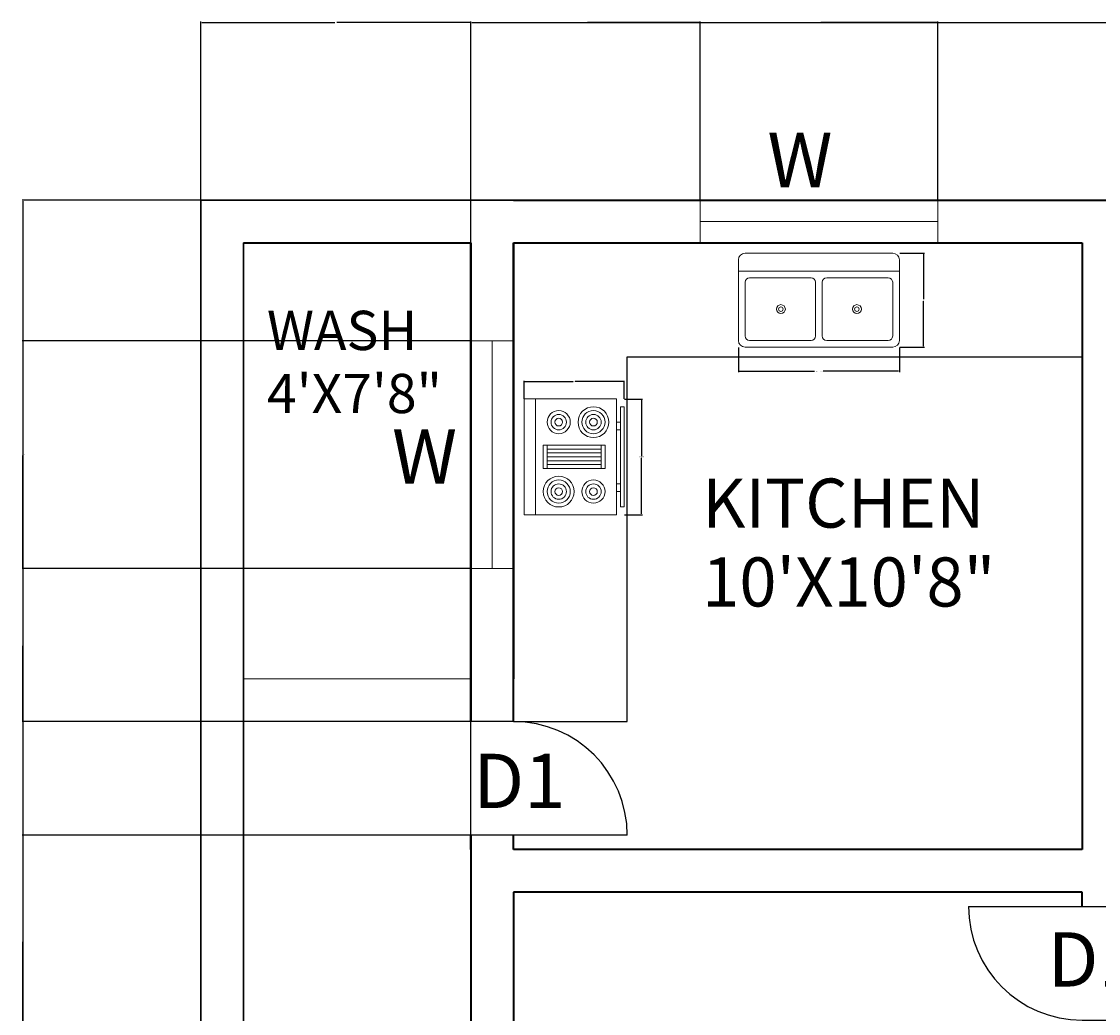
# Model space of a CAD drawing. Units: feet. Extents: x 1889 to 2708, y 1752 to 2375.
# Tile 3 of 5: x 1889 to 2116, y 2166 to 2375. Entities that reach past the tile are written whole.
import ezdxf

# ---------------------------------------------------------------- set-up
doc = ezdxf.new("R2010")
doc.units = ezdxf.units.FT
for name, color, linetype, lineweight in [('A-ANNO-DIMS', 2, 'Continuous', 18), ('A-ANNO-TEXT', 7, 'Continuous', 18), ('A-AREA-IDEN', 7, 'Continuous', 18), ('A-DOOR', 3, 'Continuous', 25), ('A-EQPM', 9, 'Continuous', 18), ('A-FLOR-CASE', 9, 'Continuous', 25), ('A-FLOR-FIXT', 8, 'Continuous', 18), ('A-GLAZ', 4, 'Continuous', 18), ('A-WALL', 7, 'Continuous', 35), ('C-PROP', 7, 'Continuous', 30), ('C-SITE', 94, 'Continuous', 18)]:
    doc.layers.add(name, color=color, linetype=linetype, lineweight=lineweight)
doc.styles.get("Standard").update_dxf_attribs({"font": 'arial.ttf'})
doc.dimstyles.get("Standard").update_dxf_attribs({"dimtxt": 0.18, "dimasz": 0.18, "dimexe": 0.18, "dimexo": 0.0625, "dimgap": 0.09, "dimtad": 0, "dimtih": 1, "dimtoh": 1, "dimdec": 4, "dimzin": 0, "dimdsep": 46, "dimtxsty": 'Standard', "dimcen": 0.09, "dimadec": 0, "dimazin": 0, "dimtfac": 1, "dimtdec": 4, "dimtofl": 0, "dimtmove": 0, "dimatfit": 3, "dimfxl": 1, "dimtolj": 1, "dimtzin": 0, "dimarcsym": 0})

# ---------------------------------------------------------------- blocks, each defined once
blk = doc.blocks.new('Range-Oven - 30 in top')
for p, q in [((0, -3), (30, -3)), ((12, -6), (18, -6)), ((13, -20), (13, -6)), ((14, -6), (14, -20)), ((15, -20), (15, -6)), ((16, -6), (16, -20)), ((17, -20), (17, -6)), ((18, -20), (12, -20)), ((6, -24), (6, -25)), ((8, -25), (8, -24)), ((22, -25), (22, -24)), ((24, -24), (24, -25))]:
    blk.add_line(p, q)
for points in [[(0, -24), (0, 0), (30, 0), (30, -24)], [(12, -21), (12, -5), (18, -5), (18, -21)], [(2, -26), (2, -25), (28, -25), (28, -26)]]:
    blk.add_lwpolyline(points, close=True)
for centre, radius in [((6, -9), 4), ((6, -9), 3), ((6, -9), 2), ((6, -9), 1), ((24, -9), 3), ((24, -9), 2), ((24, -9), 1), ((6, -18), 3), ((6, -18), 2), ((24, -18), 4), ((24, -18), 3), ((24, -18), 2), ((6, -18), 1), ((24, -18), 1)]:
    blk.add_circle(centre, radius)
blk = doc.blocks.new('Sink-double - 36 in top')
for p, q in [((-18, -4), (18, -4)), ((-0.75, -18.5), (-0.75, -6.5)), ((0.75, -6.5), (0.75, -18.5))]:
    blk.add_line(p, q)
for points in [[(-16.5, 0), (16.5, 0)], [(-18, -19.5), (-18, -1.5)], [(18, -1.5), (18, -19.5)], [(-16.5, -18.5), (-16.5, -6.5)], [(-15.5, -5.5), (-1.75, -5.5)], [(1.75, -5.5), (15.5, -5.5)], [(16.5, -6.5), (16.5, -18.5)], [(16.5, -21), (-16.5, -21)], [(-1.75, -19.5), (-15.5, -19.5)], [(15.5, -19.5), (1.75, -19.5)]]:
    blk.add_lwpolyline(points)
for centre, radius in [((-8.5, -12.5), 1), ((-8.5, -12.5), 0.5), ((8.5, -12.5), 1), ((8.5, -12.5), 0.5)]:
    blk.add_circle(centre, radius)
for centre, radius, start, end in [((-16.5, -1.5), 1.5, 90, 180), ((16.5, -1.5), 1.5, 0, 90), ((-15.5, -6.5), 1, 90, 180), ((-1.75, -6.5), 1, 0, 90), ((1.75, -6.5), 1, 90, 180), ((15.5, -6.5), 1, 0, 90), ((-15.5, -18.5), 1, 180, 270), ((-1.75, -18.5), 1, 270, 0), ((1.75, -18.5), 1, 180, 270), ((15.5, -18.5), 1, 270, 0), ((-16.5, -19.5), 1.5, 180, 270), ((16.5, -19.5), 1.5, 270, 0)]:
    blk.add_arc(centre, radius, start, end)
blk = doc.blocks.new('DOOR-SWING-24')
for p, q in [((9, 24), (0, 24)), ((33, 0), (0, 0))]:
    blk.add_line(p, q)
blk.add_arc((9, 0), 24, 0, 90)
blk = doc.blocks.new('*D27')
at = {"layer": 'A-ANNO-DIMS', "color": 0, "lineweight": -2, "transparency": 16777216}
for p, q in [((2016.29, 2295.67), (2020.07, 2295.67)), ((2019.89, 2295.49), (2019.89, 2283.65)), ((2019.89, 2271.43), (2019.89, 2283.28)), ((2016.29, 2271.25), (2020.07, 2271.25))]:
    blk.add_line(p, q, dxfattribs=at)
at = {"layer": 'A-ANNO-DIMS', "color": 0, "transparency": 16777216}
for points in [[(2019.86, 2295.49), (2019.92, 2295.49), (2019.89, 2295.67)], [(2019.86, 2271.43), (2019.92, 2271.43), (2019.89, 2271.25)]]:
    blk.add_solid(points, dxfattribs=at)
at = {"layer": 'Defpoints', "color": 0, "transparency": 16777216}
for p in [(2016.23, 2295.67), (2019.89, 2295.67), (2016.23, 2271.25)]:
    blk.add_point(p, dxfattribs=at)
at = {"layer": 'A-ANNO-DIMS', "color": 0, "transparency": 16777216, "insert": (2019.89, 2283.46), "char_height": 0.18, "attachment_point": 5}
blk.add_mtext('\\A1;HOB 24', dxfattribs=at)
blk = doc.blocks.new('*D28')
at = {"layer": 'A-ANNO-DIMS', "color": 0, "lineweight": -2, "transparency": 16777216}
for p, q in [((1995.07, 2295.73), (1995.07, 2299.51)), ((1995.25, 2299.33), (2005.44, 2299.33)), ((2016.05, 2299.33), (2005.85, 2299.33)), ((2016.23, 2295.73), (2016.23, 2299.51))]:
    blk.add_line(p, q, dxfattribs=at)
at = {"layer": 'A-ANNO-DIMS', "color": 0, "transparency": 16777216}
for points in [[(1995.25, 2299.36), (1995.25, 2299.3), (1995.07, 2299.33)], [(2016.05, 2299.36), (2016.05, 2299.3), (2016.23, 2299.33)]]:
    blk.add_solid(points, dxfattribs=at)
at = {"layer": 'Defpoints', "color": 0, "transparency": 16777216}
for p in [(1995.07, 2299.33), (1995.07, 2295.67), (2016.23, 2295.67)]:
    blk.add_point(p, dxfattribs=at)
at = {"layer": 'A-ANNO-DIMS', "color": 0, "transparency": 16777216, "insert": (2005.65, 2299.33), "char_height": 0.18, "attachment_point": 5}
blk.add_mtext('\\A1;21', dxfattribs=at)
blk = doc.blocks.new('*D33')
at = {"layer": 'A-ANNO-DIMS', "color": 0, "lineweight": -2, "transparency": 16777216}
for p, q in [((2040.31, 2306.55), (2040.31, 2301.34)), ((2074.29, 2306.55), (2074.29, 2301.34)), ((2040.49, 2301.52), (2056.4, 2301.52)), ((2074.11, 2301.52), (2058.21, 2301.52))]:
    blk.add_line(p, q, dxfattribs=at)
at = {"layer": 'A-ANNO-DIMS', "color": 0, "transparency": 16777216}
for points in [[(2040.49, 2301.55), (2040.49, 2301.49), (2040.31, 2301.52)], [(2074.11, 2301.55), (2074.11, 2301.49), (2074.29, 2301.52)]]:
    blk.add_solid(points, dxfattribs=at)
at = {"layer": 'Defpoints', "color": 0, "transparency": 16777216}
for p in [(2040.31, 2306.61), (2074.29, 2306.61), (2074.29, 2301.52)]:
    blk.add_point(p, dxfattribs=at)
at = {"layer": 'A-ANNO-DIMS', "color": 0, "transparency": 16777216, "insert": (2057.3, 2301.52), "char_height": 0.18, "attachment_point": 5}
blk.add_mtext('\\A1;TWIN SINK 34', dxfattribs=at)
blk = doc.blocks.new('*D34')
at = {"layer": 'A-ANNO-DIMS', "color": 0, "lineweight": -2, "transparency": 16777216}
for p, q in [((2074.35, 2326.44), (2079.57, 2326.44)), ((2079.39, 2326.26), (2079.39, 2316.71)), ((2079.39, 2306.79), (2079.39, 2316.34)), ((2074.35, 2306.61), (2079.57, 2306.61))]:
    blk.add_line(p, q, dxfattribs=at)
at = {"layer": 'A-ANNO-DIMS', "color": 0, "transparency": 16777216}
for points in [[(2079.36, 2326.26), (2079.42, 2326.26), (2079.39, 2326.44)], [(2079.36, 2306.79), (2079.42, 2306.79), (2079.39, 2306.61)]]:
    blk.add_solid(points, dxfattribs=at)
at = {"layer": 'Defpoints', "color": 0, "transparency": 16777216}
for p in [(2074.29, 2326.44), (2079.39, 2326.44), (2074.29, 2306.61)]:
    blk.add_point(p, dxfattribs=at)
at = {"layer": 'A-ANNO-DIMS', "color": 0, "transparency": 16777216, "insert": (2079.39, 2316.53), "char_height": 0.18, "attachment_point": 5}
blk.add_mtext('\\A1;20', dxfattribs=at)
blk = doc.blocks.new('*D35')
at = {"layer": 'A-ANNO-DIMS', "color": 0, "lineweight": -2, "transparency": 16777216}
for p, q in [((1926.86, 2337.66), (1926.86, 2375.33)), ((1983.86, 2328.66), (1983.86, 2375.33)), ((1927.04, 2375.15), (1955.15, 2375.15)), ((1983.68, 2375.15), (1955.58, 2375.15))]:
    blk.add_line(p, q, dxfattribs=at)
at = {"layer": 'A-ANNO-DIMS', "color": 0, "transparency": 16777216}
for points in [[(1927.04, 2375.18), (1927.04, 2375.12), (1926.86, 2375.15)], [(1983.68, 2375.18), (1983.68, 2375.12), (1983.86, 2375.15)]]:
    blk.add_solid(points, dxfattribs=at)
at = {"layer": 'Defpoints', "color": 0, "transparency": 16777216}
for p in [(1983.86, 2375.15), (1926.86, 2337.6), (1983.86, 2328.6)]:
    blk.add_point(p, dxfattribs=at)
at = {"layer": 'A-ANNO-DIMS', "color": 0, "transparency": 16777216, "insert": (1955.36, 2375.15), "char_height": 0.18, "attachment_point": 5}
blk.add_mtext('\\A1;57', dxfattribs=at)
blk = doc.blocks.new('*D36')
at = {"layer": 'A-ANNO-DIMS', "color": 0, "lineweight": -2, "transparency": 16777216}
for p, q in [((1983.86, 2328.66), (1983.86, 2375.33)), ((2032.22, 2337.66), (2032.22, 2375.33)), ((1984.04, 2375.15), (2007.64, 2375.15)), ((2032.04, 2375.15), (2008.44, 2375.15))]:
    blk.add_line(p, q, dxfattribs=at)
at = {"layer": 'A-ANNO-DIMS', "color": 0, "transparency": 16777216}
for points in [[(1984.04, 2375.18), (1984.04, 2375.12), (1983.86, 2375.15)], [(2032.04, 2375.18), (2032.04, 2375.12), (2032.22, 2375.15)]]:
    blk.add_solid(points, dxfattribs=at)
at = {"layer": 'Defpoints', "color": 0, "transparency": 16777216}
for p in [(2032.22, 2375.15), (2032.22, 2337.6), (1983.86, 2328.6)]:
    blk.add_point(p, dxfattribs=at)
at = {"layer": 'A-ANNO-DIMS', "color": 0, "transparency": 16777216, "insert": (2008.04, 2375.15), "char_height": 0.18, "attachment_point": 5}
blk.add_mtext('\\A1;48.35', dxfattribs=at)
blk = doc.blocks.new('*D37')
at = {"layer": 'A-ANNO-DIMS', "color": 0, "lineweight": -2, "transparency": 16777216}
for p, q in [((2032.22, 2337.66), (2032.22, 2375.33)), ((2082.41, 2337.66), (2082.41, 2375.33)), ((2032.4, 2375.15), (2056.92, 2375.15)), ((2082.23, 2375.15), (2057.71, 2375.15))]:
    blk.add_line(p, q, dxfattribs=at)
at = {"layer": 'A-ANNO-DIMS', "color": 0, "transparency": 16777216}
for points in [[(2032.4, 2375.18), (2032.4, 2375.12), (2032.22, 2375.15)], [(2082.23, 2375.18), (2082.23, 2375.12), (2082.41, 2375.15)]]:
    blk.add_solid(points, dxfattribs=at)
at = {"layer": 'Defpoints', "color": 0, "transparency": 16777216}
for p in [(2082.41, 2375.15), (2032.22, 2337.6), (2082.41, 2337.6)]:
    blk.add_point(p, dxfattribs=at)
at = {"layer": 'A-ANNO-DIMS', "color": 0, "transparency": 16777216, "insert": (2057.31, 2375.15), "char_height": 0.18, "attachment_point": 5}
blk.add_mtext('\\A1;50.19', dxfattribs=at)
blk = doc.blocks.new('*D38')
at = {"layer": 'A-ANNO-DIMS', "color": 0, "lineweight": -2, "transparency": 16777216}
for p, q in [((2082.41, 2337.66), (2082.41, 2375.33)), ((2344.63, 2337.66), (2344.63, 2375.33)), ((2082.59, 2375.15), (2213.05, 2375.15)), ((2344.45, 2375.15), (2213.98, 2375.15))]:
    blk.add_line(p, q, dxfattribs=at)
at = {"layer": 'A-ANNO-DIMS', "color": 0, "transparency": 16777216}
for points in [[(2082.59, 2375.18), (2082.59, 2375.12), (2082.41, 2375.15)], [(2344.45, 2375.18), (2344.45, 2375.12), (2344.63, 2375.15)]]:
    blk.add_solid(points, dxfattribs=at)
at = {"layer": 'Defpoints', "color": 0, "transparency": 16777216}
for p in [(2344.63, 2375.15), (2082.41, 2337.6), (2344.63, 2337.6)]:
    blk.add_point(p, dxfattribs=at)
at = {"layer": 'A-ANNO-DIMS', "color": 0, "transparency": 16777216, "insert": (2213.52, 2375.15), "char_height": 0.18, "attachment_point": 5}
blk.add_mtext('\\A1;262.23', dxfattribs=at)
blk = doc.blocks.new('*D46')
at = {"layer": 'A-ANNO-DIMS', "color": 0, "lineweight": -2, "transparency": 16777216}
for p, q in [((1926.8, 2337.6), (1889.13, 2337.6)), ((1889.31, 2337.42), (1889.31, 2121.28)), ((1889.31, 1904.78), (1889.31, 2120.92)), ((1983.8, 1904.6), (1889.13, 1904.6))]:
    blk.add_line(p, q, dxfattribs=at)
at = {"layer": 'A-ANNO-DIMS', "color": 0, "transparency": 16777216}
for points in [[(1889.28, 2337.42), (1889.34, 2337.42), (1889.31, 2337.6)], [(1889.28, 1904.78), (1889.34, 1904.78), (1889.31, 1904.6)]]:
    blk.add_solid(points, dxfattribs=at)
at = {"layer": 'Defpoints', "color": 0, "transparency": 16777216}
for p in [(1889.31, 2337.6), (1926.86, 2337.6), (1983.86, 1904.6)]:
    blk.add_point(p, dxfattribs=at)
at = {"layer": 'A-ANNO-DIMS', "color": 0, "transparency": 16777216, "insert": (1889.31, 2121.1), "char_height": 0.18, "attachment_point": 5}
blk.add_mtext('\\A1;433', dxfattribs=at)
blk = doc.blocks.new('*D48')
at = {"layer": 'A-ANNO-DIMS', "color": 0, "lineweight": -2, "transparency": 16777216}
for p, q in [((1983.86, 1820.66), (1983.86, 2375.33)), ((2432.86, 1820.66), (2432.86, 2375.33)), ((1984.04, 2375.15), (2208.07, 2375.15)), ((2432.68, 2375.15), (2208.66, 2375.15))]:
    blk.add_line(p, q, dxfattribs=at)
at = {"layer": 'A-ANNO-DIMS', "color": 0, "transparency": 16777216}
for points in [[(1984.04, 2375.18), (1984.04, 2375.12), (1983.86, 2375.15)], [(2432.68, 2375.18), (2432.68, 2375.12), (2432.86, 2375.15)]]:
    blk.add_solid(points, dxfattribs=at)
at = {"layer": 'Defpoints', "color": 0, "transparency": 16777216}
for p in [(2432.86, 2375.15), (1983.86, 1820.6), (2432.86, 1820.6)]:
    blk.add_point(p, dxfattribs=at)
at = {"layer": 'A-ANNO-DIMS', "color": 0, "transparency": 16777216, "insert": (2208.36, 2375.15), "char_height": 0.18, "attachment_point": 5}
blk.add_mtext('\\A1;449', dxfattribs=at)
blk = doc.blocks.new('*D55')
at = {"layer": 'A-ANNO-DIMS', "color": 0, "lineweight": -2, "transparency": 16777216}
for p, q in [((1983.8, 2203.6), (1889.13, 2203.6)), ((1889.31, 2203.42), (1889.31, 2181.48)), ((1889.31, 2159.18), (1889.31, 2181.12)), ((1983.8, 2159), (1889.13, 2159))]:
    blk.add_line(p, q, dxfattribs=at)
at = {"layer": 'A-ANNO-DIMS', "color": 0, "transparency": 16777216}
for points in [[(1889.28, 2203.42), (1889.34, 2203.42), (1889.31, 2203.6)], [(1889.28, 2159.18), (1889.34, 2159.18), (1889.31, 2159)]]:
    blk.add_solid(points, dxfattribs=at)
at = {"layer": 'Defpoints', "color": 0, "transparency": 16777216}
for p in [(1889.31, 2203.6), (1983.86, 2203.6), (1983.86, 2159)]:
    blk.add_point(p, dxfattribs=at)
at = {"layer": 'A-ANNO-DIMS', "color": 0, "transparency": 16777216, "insert": (1889.31, 2181.3), "char_height": 0.18, "attachment_point": 5}
blk.add_mtext('\\A1;44.6', dxfattribs=at)
blk = doc.blocks.new('*D56')
at = {"layer": 'A-ANNO-DIMS', "color": 0, "lineweight": -2, "transparency": 16777216}
for p, q in [((1983.8, 2259.92), (1889.13, 2259.92)), ((1889.31, 2259.74), (1889.31, 2243.94)), ((1889.31, 2227.78), (1889.31, 2243.58)), ((1983.8, 2227.6), (1889.13, 2227.6))]:
    blk.add_line(p, q, dxfattribs=at)
at = {"layer": 'A-ANNO-DIMS', "color": 0, "transparency": 16777216}
for points in [[(1889.28, 2259.74), (1889.34, 2259.74), (1889.31, 2259.92)], [(1889.28, 2227.78), (1889.34, 2227.78), (1889.31, 2227.6)]]:
    blk.add_solid(points, dxfattribs=at)
at = {"layer": 'Defpoints', "color": 0, "transparency": 16777216}
for p in [(1889.31, 2259.92), (1983.86, 2259.92), (1983.86, 2227.6)]:
    blk.add_point(p, dxfattribs=at)
at = {"layer": 'A-ANNO-DIMS', "color": 0, "transparency": 16777216, "insert": (1889.31, 2243.76), "char_height": 0.18, "attachment_point": 5}
blk.add_mtext('\\A1;32.32', dxfattribs=at)
blk = doc.blocks.new('*D57')
at = {"layer": 'A-ANNO-DIMS', "color": 0, "lineweight": -2, "transparency": 16777216}
for p, q in [((1983.8, 2307.98), (1889.13, 2307.98)), ((1889.31, 2307.8), (1889.31, 2284.13)), ((1889.31, 2260.1), (1889.31, 2283.77)), ((1983.8, 2259.92), (1889.13, 2259.92))]:
    blk.add_line(p, q, dxfattribs=at)
at = {"layer": 'A-ANNO-DIMS', "color": 0, "transparency": 16777216}
for points in [[(1889.28, 2307.8), (1889.34, 2307.8), (1889.31, 2307.98)], [(1889.28, 2260.1), (1889.34, 2260.1), (1889.31, 2259.92)]]:
    blk.add_solid(points, dxfattribs=at)
at = {"layer": 'Defpoints', "color": 0, "transparency": 16777216}
for p in [(1889.31, 2307.98), (1983.86, 2307.98), (1983.86, 2259.92)]:
    blk.add_point(p, dxfattribs=at)
at = {"layer": 'A-ANNO-DIMS', "color": 0, "transparency": 16777216, "insert": (1889.31, 2283.95), "char_height": 0.18, "attachment_point": 5}
blk.add_mtext('\\A1;48.06', dxfattribs=at)

msp = doc.modelspace()

# ---------------------------------------------------------------- linework, layer by layer
at = {"layer": 'A-FLOR-CASE'}
for p, q in [((2016.8644, 2304.5988), (2112.8644, 2304.5988)), ((2016.8644, 2227.5988), (2016.8644, 2304.5988)), ((1992.8644, 2227.5988), (2016.8644, 2227.5988))]:
    msp.add_line(p, q, dxfattribs=at)
at = {"layer": 'A-GLAZ'}
for p, q in [((2032.217, 2337.5988), (2032.217, 2328.5988)), ((2082.4064, 2337.5988), (2082.4064, 2328.5988)), ((2032.217, 2333.0988), (2082.4064, 2333.0988)), ((1983.8644, 2307.9791), (1992.8644, 2307.9791)), ((1988.3644, 2307.9791), (1988.3644, 2259.9212)), ((1983.8644, 2259.9212), (1992.8644, 2259.9212))]:
    msp.add_line(p, q, dxfattribs=at)
at = {"layer": 'A-WALL'}
for p, q in [((1992.8644, 2337.5988), (2669.8644, 2337.5988)), ((1935.8644, 2328.5988), (1983.8644, 2328.5988)), ((1983.8644, 2328.5988), (1983.8644, 2236.5988)), ((1983.8644, 2227.5988), (1983.8644, 2328.5988)), ((1992.8644, 2328.5988), (1992.8644, 2236.5988)), ((1992.8644, 2328.5988), (2112.8644, 2328.5988)), ((1992.8644, 2227.5988), (1992.8644, 2328.5988)), ((2112.8644, 2328.5988), (2112.8644, 2200.5988)), ((1983.8644, 2236.5988), (1983.8644, 2227.5988)), ((1983.8644, 2236.5988), (1983.8644, 2227.5988)), ((1983.8644, 2236.5988), (1983.8644, 2227.5988)), ((1983.8644, 2200.5988), (1983.8644, 2203.5988)), ((1983.8644, 2203.5988), (1983.8644, 1904.5988)), ((1983.8644, 2203.5988), (1983.8644, 1974.5988)), ((1983.8644, 2203.5988), (1983.8644, 2039.5988)), ((1992.8644, 2200.5988), (1992.8644, 2203.5988)), ((2112.8644, 2200.5988), (1992.8644, 2200.5988)), ((2112.8644, 2191.5988), (1992.8644, 2191.5988)), ((1992.8644, 2191.5988), (1992.8644, 2039.5988)), ((2112.8644, 2188.5988), (2112.8644, 2191.5988))]:
    msp.add_line(p, q, dxfattribs=at)
at = {"layer": 'C-PROP'}
for p, q in [((1926.8644, 2337.5988), (2669.8644, 2337.5988)), ((1926.8644, 2236.5988), (1926.8644, 2337.5988)), ((1935.8644, 1811.5988), (1935.8644, 2328.5988)), ((1926.8644, 2236.5988), (1926.8644, 1811.5988))]:
    msp.add_line(p, q, dxfattribs=at)
at = {"layer": 'C-SITE'}
msp.add_line((1983.8644, 2236.5988), (1935.8644, 2236.5988), dxfattribs=at)

# ---------------------------------------------------------------- block references
at = {"layer": 'A-DOOR'}
msp.add_blockref('DOOR-SWING-24', (1983.864, 2203.599), dxfattribs=at)
at = {"layer": 'A-DOOR', "rotation": 180}
msp.add_blockref('DOOR-SWING-24', (2121.8649, 2188.5986), dxfattribs=at)
at = {"layer": 'A-EQPM', "xscale": 0.8139749521299275, "yscale": 0.8139749521299275, "zscale": 0.8139749521299275, "rotation": 90}
msp.add_blockref('Range-Oven - 30 in top', (1995.0661, 2271.2526), dxfattribs=at)
at = {"layer": 'A-FLOR-FIXT', "xscale": 0.9438809803131618, "yscale": 0.9438809803131618, "zscale": 0.9438809803131618}
msp.add_blockref('Sink-double - 36 in top', (2057.3006, 2326.4365), dxfattribs=at)

# ---------------------------------------------------------------- texts
at = {"layer": 'A-ANNO-TEXT'}
for s, height, p in [('W', 11.4692, (2046.4356, 2340.3733)), ('W', 11.4692, (1967.2097, 2277.7906)), ('D1', 11.46921, (1984.3378, 2209.3351)), ('D1', 11.46921, (2105.5594, 2171.6646))]:
    msp.add_text(s, height=height, dxfattribs=at).set_placement(p)
at = {"layer": 'A-AREA-IDEN'}
for s, height, p in [('WASH', 8.28631, (1940.8052, 2306.0014)), ('4\'X7\'8"', 8.28631, (1940.8052, 2292.6901)), ('KITCHEN', 10.35971, (2032.6711, 2268.5215)), ('10\'X10\'8"', 10.35971, (2032.6711, 2251.8795))]:
    msp.add_text(s, height=height, dxfattribs=at).set_placement(p)

# ---------------------------------------------------------------- dimensions: what is measured, and where the dimension line sits
at = {"layer": 'A-ANNO-DIMS'}
for base, p1, p2, override, picture, middle in [((1983.8644, 2375.1488), (1926.8644, 2337.5988), (1983.8644, 2328.5988), {"dimdec": 0, "dimlfac": 1, "dimrnd": 0, "dimzin": 0, "dimdsep": 46, "dimlunit": 2}, '*D35', (1955.3644, 2375.1488)), ((2032.217, 2375.1488), (1983.8644, 2328.5988), (2032.217, 2337.5988), {"dimdec": 2, "dimlfac": 1, "dimrnd": 0, "dimzin": 0, "dimdsep": 46, "dimlunit": 2}, '*D36', (2008.0407, 2375.1488)), ((2432.8644, 2375.1488), (1983.8644, 1820.5988), (2432.8644, 1820.5988), {"dimdec": 0, "dimlfac": 1, "dimrnd": 0, "dimzin": 0, "dimdsep": 46, "dimlunit": 2}, '*D48', (2208.3644, 2375.1488)), ((2082.4064, 2375.1488), (2032.217, 2337.5988), (2082.4064, 2337.5988), {"dimdec": 2, "dimlfac": 1, "dimrnd": 0, "dimzin": 0, "dimdsep": 46, "dimlunit": 2}, '*D37', (2057.3117, 2375.1488)), ((2344.6329, 2375.1488), (2082.4064, 2337.5988), (2344.6329, 2337.5988), {"dimdec": 2, "dimlfac": 1, "dimrnd": 0, "dimzin": 0, "dimdsep": 46, "dimlunit": 2}, '*D38', (2213.5196, 2375.1488))]:
    dim = msp.add_linear_dim(base=base, p1=p1, p2=p2, dimstyle='Standard', override=override, dxfattribs=at)
    dim.commit()
    dim.dimension.update_dxf_attribs({"geometry": picture, "text_midpoint": middle})
for base, p1, p2, angle, override, picture, middle in [((1889.3144, 2337.5988), (1983.8644, 1904.5988), (1926.8644, 2337.5988), 90, {"dimdec": 0, "dimlfac": 1, "dimrnd": 0, "dimzin": 0, "dimdsep": 46, "dimlunit": 2}, '*D46', (1889.3144, 2121.0988)), ((2079.3874, 2326.4365), (2074.2905, 2306.615), (2074.2905, 2326.4365), 90, {"dimdec": 0, "dimlfac": 1, "dimrnd": 0, "dimzin": 0, "dimdsep": 46, "dimlunit": 2}, '*D34', (2079.3874, 2316.5257)), ((1889.3144, 2307.9791), (1983.8644, 2259.9212), (1983.8644, 2307.9791), 90, {"dimdec": 2, "dimlfac": 1, "dimrnd": 0, "dimzin": 0, "dimdsep": 46, "dimlunit": 2}, '*D57', (1889.3144, 2283.9502)), ((1995.0661, 2299.3348), (2016.2295, 2295.6719), (1995.0661, 2295.6719), 180, {"dimdec": 0, "dimlfac": 1, "dimrnd": 0, "dimzin": 0, "dimdsep": 46, "dimlunit": 2}, '*D28', (2005.6478, 2299.3348)), ((1889.3144, 2259.9212), (1983.8644, 2227.5988), (1983.8644, 2259.9212), 90, {"dimdec": 2, "dimlfac": 1, "dimrnd": 0, "dimzin": 0, "dimdsep": 46, "dimlunit": 2}, '*D56', (1889.3144, 2243.76)), ((1889.3144, 2203.5988), (1983.8644, 2158.9974), (1983.8644, 2203.5988), 90, {"dimdec": 1, "dimlfac": 1, "dimrnd": 0, "dimzin": 0, "dimdsep": 46, "dimlunit": 2}, '*D55', (1889.3144, 2181.2981))]:
    dim = msp.add_linear_dim(base=base, p1=p1, p2=p2, angle=angle, dimstyle='Standard', override=override, dxfattribs=at)
    dim.commit()
    dim.dimension.update_dxf_attribs({"geometry": picture, "text_midpoint": middle})
dim = msp.add_linear_dim(base=(2074.2905, 2301.518), p1=(2040.3108, 2306.615), p2=(2074.2905, 2306.615), text='TWIN SINK <>', dimstyle='Standard', override={"dimdec": 0, "dimlfac": 1, "dimrnd": 0, "dimzin": 0, "dimdsep": 46, "dimlunit": 2}, dxfattribs=at)
dim.commit()
dim.dimension.update_dxf_attribs({"geometry": '*D33', "text_midpoint": (2057.3006, 2301.518)})
dim = msp.add_linear_dim(base=(2019.8924, 2295.6719), p1=(2016.2295, 2271.2526), p2=(2016.2295, 2295.6719), angle=90, text='HOB <>', dimstyle='Standard', override={"dimdec": 0, "dimlfac": 1, "dimrnd": 0, "dimzin": 0, "dimdsep": 46, "dimlunit": 2}, dxfattribs=at)
dim.commit()
dim.dimension.update_dxf_attribs({"geometry": '*D27', "text_midpoint": (2019.8924, 2283.4623)})

doc.saveas('drawing.dxf')
